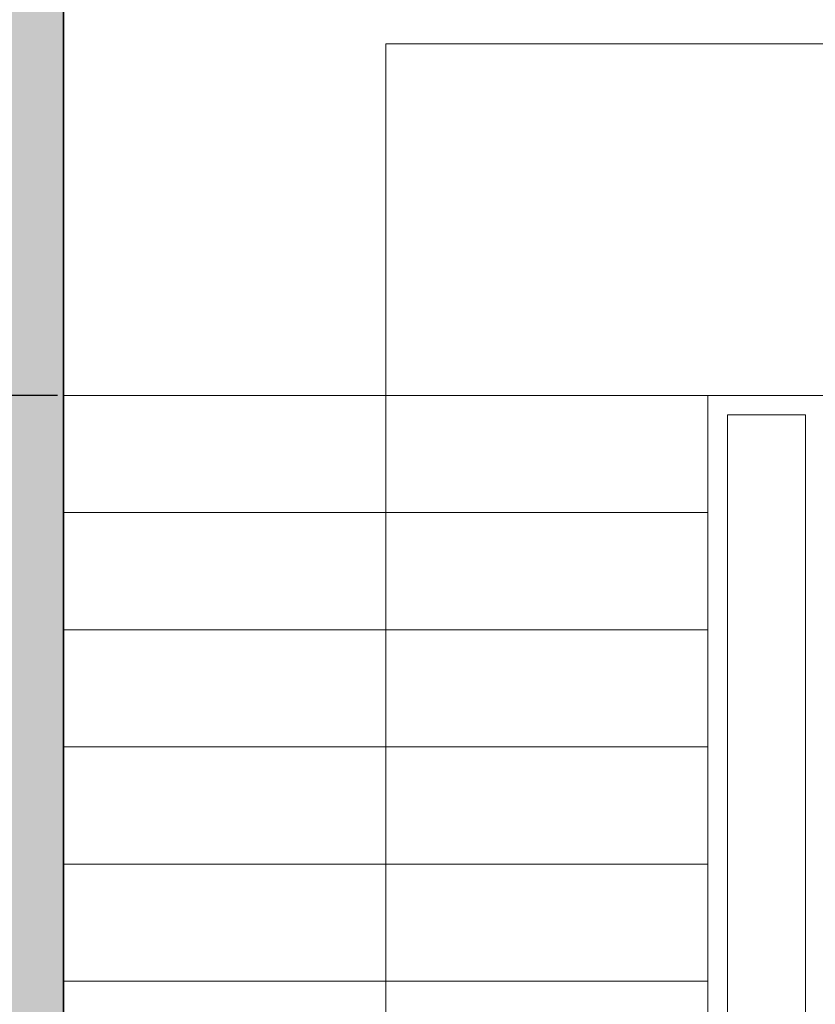
# Model space of a CAD drawing. Units: inches. Extents: x 2083 to 3317, y 1141 to 2115.
# Tile 256 of 256: x 2600 to 2682, y 1877 to 1978. Entities that reach past the tile are written whole.
import ezdxf

# ---------------------------------------------------------------- set-up
doc = ezdxf.new("R2010")
doc.units = ezdxf.units.IN
for name, color, linetype, lineweight in [('A-ANNO-DIMS', 2, 'Continuous', 18), ('A-ANNO-SYMB', 7, 'Continuous', 13), ('A-FLOR-STRS', 7, 'Continuous', 18), ('A-WALL', 7, 'Continuous', 35)]:
    doc.layers.add(name, color=color, linetype=linetype, lineweight=lineweight)
doc.layers.add('A-WALL-PATT', color=251, linetype='Continuous', lineweight=13, true_color=0x636466)
doc.styles.get("Standard").update_dxf_attribs({"font": 'arial.ttf'})
doc.dimstyles.new('ISO-25', dxfattribs={"dimtxt": 12, "dimasz": 12, "dimexe": 1.25, "dimexo": 0.625, "dimtad": 1, "dimlunit": 3, "dimtxsty": 'Standard', "dimcen": 2.5, "dimadec": 0, "dimazin": 0, "dimtfac": 1, "dimtmove": 0, "dimatfit": 3, "dimfxl": 1, "dimarcsym": 0})

# ---------------------------------------------------------------- blocks, each defined once
blk = doc.blocks.new('*D50')
at = {"layer": 'A-ANNO-DIMS', "color": 0, "lineweight": -2, "transparency": 16777216}
for p, q in [((2604.33, 1939.76), (2551.36, 1939.76)), ((2552.61, 1807.76), (2552.61, 1927.76)), ((2604.33, 1795.76), (2551.36, 1795.76))]:
    blk.add_line(p, q, dxfattribs=at)
at = {"layer": 'A-ANNO-DIMS', "color": 0, "transparency": 16777216}
for points in [[(2550.61, 1927.76), (2554.61, 1927.76), (2552.61, 1939.76)], [(2550.61, 1807.76), (2554.61, 1807.76), (2552.61, 1795.76)]]:
    blk.add_solid(points, dxfattribs=at)
at = {"layer": 'Defpoints', "color": 0, "transparency": 16777216}
for p in [(2552.61, 1939.76), (2604.96, 1939.76), (2604.96, 1795.76)]:
    blk.add_point(p, dxfattribs=at)
at = {"layer": 'A-ANNO-DIMS', "color": 0, "transparency": 16777216, "insert": (2545.86, 1867.76), "char_height": 12, "attachment_point": 5, "rotation": 90}
blk.add_mtext('12\'-0"', dxfattribs=at)
blk = doc.blocks.new('*D51')
at = {"layer": 'A-ANNO-DIMS', "color": 0, "lineweight": -2, "transparency": 16777216}
for p, q in [((2604.33, 2011.76), (2551.36, 2011.76)), ((2552.61, 1951.76), (2552.61, 1999.76)), ((2604.33, 1939.76), (2551.36, 1939.76))]:
    blk.add_line(p, q, dxfattribs=at)
at = {"layer": 'A-ANNO-DIMS', "color": 0, "transparency": 16777216}
for points in [[(2550.61, 1999.76), (2554.61, 1999.76), (2552.61, 2011.76)], [(2550.61, 1951.76), (2554.61, 1951.76), (2552.61, 1939.76)]]:
    blk.add_solid(points, dxfattribs=at)
at = {"layer": 'Defpoints', "color": 0, "transparency": 16777216}
for p in [(2552.61, 2011.76), (2604.96, 2011.76), (2604.96, 1939.76)]:
    blk.add_point(p, dxfattribs=at)
at = {"layer": 'A-ANNO-DIMS', "color": 0, "transparency": 16777216, "insert": (2545.86, 1975.76), "char_height": 12, "attachment_point": 5, "rotation": 90}
blk.add_mtext('6\'-0"', dxfattribs=at)

msp = doc.modelspace()

# ---------------------------------------------------------------- hatches: boundary and pattern name
at = {"layer": 'A-WALL-PATT'}
h = msp.add_hatch(color=256, dxfattribs=at)
h.dxf.hatch_style = 1
h.paths.add_polyline_path([(3126.96, 2020.761), (2748.96, 2020.761), (2604.96, 2020.761), (2226.96, 2020.761), (2226.96, 1702.761), (2466.96, 1702.761), (2466.96, 1582.761), (2418.96, 1582.761), (2418.96, 1477.761), (2226.96, 1477.761), (2226.96, 1263.261), (2544.96, 1263.261), (2544.96, 1411.761), (2604.96, 1411.761), (2685.96, 1411.761), (2685.96, 1420.761), (2604.96, 1420.761), (2604.96, 1573.761), (2604.96, 1702.761), (2604.96, 2011.761), (2748.96, 2011.761), (2748.96, 1702.761), (2862.96, 1702.761), (2862.96, 1621.761), (2871.96, 1621.761), (2871.96, 1702.761), (2883.96, 1702.761), (2883.96, 1706.939, -0.0264593), (2883.96, 1711.761), (2757.96, 1711.761), (2757.96, 1807.761), (2787.96, 1807.761), (2787.96, 1812.261), (2757.96, 1812.261), (2757.96, 2011.761), (2877.96, 2011.761), (2877.96, 1812.261), (2847.96, 1812.261), (2847.96, 1807.761), (2889.836, 1807.761), (2889.836, 1812.261), (2882.46, 1812.261), (2882.46, 2011.761), (3117.96, 2011.761), (3117.96, 1812.261), (2937.836, 1812.261), (2937.836, 1807.761), (2995.71, 1807.761), (2995.71, 1796.118), (3000.21, 1796.118), (3000.21, 1807.761), (3117.96, 1807.761), (3117.96, 1711.761), (3000.21, 1711.761), (3000.21, 1760.118), (2998.573, 1760.118, -0.020711), (2995.71, 1760.118), (2995.71, 1711.761), (2931.96, 1711.761), (2931.96, 1702.761), (3126.96, 1702.761)])
h.paths.add_polyline_path([(2471.46, 2011.761), (2471.46, 1810.011), (2462.717, 1810.011), (2462.717, 1805.511), (2505.96, 1805.511), (2505.96, 1810.011), (2475.96, 1810.011), (2475.96, 2011.761), (2595.96, 2011.761), (2595.96, 1810.011), (2565.96, 1810.011), (2565.96, 1805.511), (2595.96, 1805.511), (2595.96, 1711.761), (2235.96, 1711.761), (2235.96, 1805.511), (2353.71, 1805.511), (2353.71, 1796.054), (2358.21, 1796.054), (2358.21, 1805.511), (2414.717, 1805.511), (2414.717, 1810.011), (2235.96, 1810.011), (2235.96, 2011.761)], flags=16)
h.paths.add_polyline_path([(2270.205, 1994.61), (2270.205, 1970.61), (2246.205, 1970.61), (2246.205, 1994.61)], flags=0)
edge = h.paths.add_edge_path(flags=0)
edge.add_ellipse((2332.027, 1899.798), major_axis=(-3.043, 3.043), ratio=0.1682525, start_angle=-161.33217, end_angle=-156.30711, ccw=False)
edge.add_ellipse((2333.082, 1898.744), major_axis=(-1.055, 1.055), ratio=0.4535321, start_angle=-123.37102, end_angle=-94.15911)
edge = h.paths.add_edge_path(flags=0)
edge.add_ellipse((2332.027, 1968.876), major_axis=(3.043, 3.043), ratio=0.1682525, start_angle=18.66783, end_angle=23.69289)
edge.add_spline(control_points=[(2332.926, 1970.691), (2332.227, 1970.336), (2330.894, 1969.659), (2328.413, 1970.932), (2327.204, 1967.749), (2324.71, 1969.956), (2322.533, 1967.012), (2320.013, 1971.296), (2317.68, 1968.158), (2316.041, 1967.102), (2315.427, 1966.81)], knot_values=[0, 0, 0, 0, 2.2670587, 4.3245589, 6.6855835, 8.8786411, 11.121502, 14.300359, 17.7552837, 19.732645, 19.732645, 19.732645, 19.732645], degree=3, periodic=0)
edge.add_ellipse((2332.027, 1968.876), major_axis=(3.043, 3.043), ratio=0.1682525, start_angle=18.66783, end_angle=23.69289, ccw=False)
edge.add_ellipse((2333.082, 1969.931), major_axis=(1.055, 1.055), ratio=0.4535321, start_angle=56.62898, end_angle=85.84089, ccw=False)
edge = h.paths.add_edge_path(flags=0)
edge.add_spline(control_points=[(2296.428, 1967.988), (2293.628, 1965.336), (2287.704, 1959.727), (2299.744, 1949.996), (2294.533, 1935.669), (2290.573, 1920.604), (2293.394, 1909.974), (2296.185, 1904.967)], knot_values=[0.0991853, 0.0991853, 0.0991853, 0.0991853, 0.3453009, 0.6198217, 0.9826526, 1.3860932, 1.8105546, 1.8105546, 1.8105546, 1.8105546], degree=3, periodic=0)
edge.add_spline(control_points=[(2296.185, 1904.967), (2297.384, 1902.619), (2298.001, 1901.949), (2298.553, 1901.468)], knot_values=[0.0062457, 0.0062457, 0.0062457, 0.0062457, 0.0554759, 0.0554759, 0.0554759, 0.0554759], degree=3, periodic=0)
edge.add_spline(control_points=[(2298.553, 1901.468), (2297.259, 1900.923), (2295.225, 1900.232), (2293.06, 1900.614), (2292.101, 1900.788), (2292.09, 1900.791)], knot_values=[0.3128349, 0.3128349, 0.3128349, 0.3128349, 0.4017797, 0.4749867, 0.4759027, 0.4759027, 0.4759027, 0.4759027], degree=3, periodic=0)
edge.add_arc((2292.794, 1904.664), 3.937, 215.4209, 259.69818, ccw=False)
edge.add_spline(control_points=[(2289.585, 1902.382), (2289.477, 1902.535), (2289.368, 1902.688), (2289.261, 1902.841)], knot_values=[0.1028719, 0.1028719, 0.1028719, 0.1028719, 0.1168958, 0.1168958, 0.1168958, 0.1168958], degree=3, periodic=0)
edge.add_spline(control_points=[(2289.261, 1902.841), (2288.687, 1902.55), (2287.64, 1902.02), (2285.881, 1901.874), (2283.853, 1901.504), (2281.72, 1899.711), (2278.467, 1899.493), (2276.157, 1901.883), (2272.259, 1899.804), (2267.778, 1901.843), (2262.244, 1900.184), (2257.415, 1901.782), (2254.318, 1900.726), (2253.178, 1900.337)], knot_values=[0, 0, 0, 0, 1.9079767, 3.4771759, 5.261074, 7.9728515, 11.6802485, 13.7179214, 16.9395917, 22.789562, 27.5025027, 33.5952153, 37.1456181, 37.1456181, 37.1456181, 37.1456181], degree=3, periodic=0)
edge.add_line((2253.178, 1900.337), (2250.244, 1902.841))
edge.add_line((2250.244, 1902.841), (2250.244, 1965.833))
edge.add_line((2250.244, 1965.833), (2253.178, 1968.337))
edge.add_spline(control_points=[(2253.178, 1968.337), (2254.318, 1967.948), (2257.415, 1966.892), (2262.244, 1968.49), (2267.778, 1966.831), (2271.527, 1968.537), (2273.876, 1967.828), (2274.207, 1967.728)], knot_values=[0, 0, 0, 0, 0.0901802, 0.2449351, 0.3646438, 0.5132331, 0.5378548, 0.5378548, 0.5378548, 0.5378548], degree=3, periodic=0)
edge.add_arc((2274.353, 1963.793), 3.937, 72.05113, 92.12795, ccw=False)
edge.add_arc((2281.297, 1985.23), 18.596, 252.05113, 288.56572)
edge.add_arc((2292.317, 1956.029), 12.646, 71.02679, 113.77822, ccw=False)
edge = h.paths.add_edge_path(flags=0)
edge.add_spline(control_points=[(2274.899, 1951.856), (2275.066, 1951.617), (2275.233, 1951.377), (2275.398, 1951.136)], knot_values=[1.4099157, 1.4099157, 1.4099157, 1.4099157, 1.4315903, 1.4315903, 1.4315903, 1.4315903], degree=3, periodic=0)
edge.add_spline(control_points=[(2275.398, 1951.136), (2275.792, 1950.562), (2276.179, 1949.984), (2276.546, 1949.397)], knot_values=[1.3582378, 1.3582378, 1.3582378, 1.3582378, 1.4099157, 1.4099157, 1.4099157, 1.4099157], degree=3, periodic=0)
edge.add_line((2276.546, 1949.397), (2277.437, 1947.862))
edge.add_spline(control_points=[(2277.437, 1947.862), (2276.304, 1945.673), (2274.64, 1942.427), (2274.632, 1938.094), (2272.799, 1930.852), (2274.356, 1943.897), (2275.948, 1947.923), (2276.546, 1949.397)], knot_values=[0.0056315, 0.0056315, 0.0056315, 0.0056315, 0.1860139, 0.2660015, 0.3570872, 0.5963902, 0.7397317, 0.7397317, 0.7397317, 0.7397317], degree=3, periodic=0)
edge.add_spline(control_points=[(2276.546, 1949.397), (2276.179, 1949.984), (2275.792, 1950.562), (2275.398, 1951.136)], knot_values=[1.3582378, 1.3582378, 1.3582378, 1.3582378, 1.4099157, 1.4099157, 1.4099157, 1.4099157], degree=3, periodic=0)
edge.add_spline(control_points=[(2275.398, 1951.136), (2274.943, 1950.08), (2274.208, 1948.025), (2273.935, 1944.851), (2272.469, 1937.627), (2273.466, 1945.696), (2274.701, 1951.059), (2274.899, 1951.856)], knot_values=[0.1043639, 0.1043639, 0.1043639, 0.1043639, 0.1896363, 0.2696239, 0.3607096, 0.6000126, 0.6446217, 0.6446217, 0.6446217, 0.6446217], degree=3, periodic=0)
h.paths.add_polyline_path([(2269.168, 1963.128, -0.3575267), (2268.171, 1960.976, -0.0925607), (2268.171, 1939.436, -0.3575267), (2269.168, 1937.285, -0.3575267), (2267.016, 1938.282, -0.1647847), (2254.686, 1938.282, -0.3575267), (2252.534, 1937.285, -0.3575267), (2253.531, 1939.436, -0.0925607), (2253.531, 1960.976, -0.3575267), (2252.534, 1963.128, -0.3575267), (2254.686, 1962.131, -0.1647847), (2267.016, 1962.131, -0.3575267)], flags=0)
h.paths.add_polyline_path([(2248.874, 1967.802), (2248.874, 1957.028), (2249.458, 1957.028), (2249.458, 1911.647), (2248.874, 1911.647), (2248.874, 1900.873), (2246.512, 1900.873, 0.1973271), (2244.15, 1902.457), (2244.15, 1966.218, 0.1973271), (2246.512, 1967.802)], flags=0)
h.paths.add_polyline_path([(2269.168, 1931.389, -0.3575267), (2268.171, 1929.238, -0.0925607), (2268.171, 1907.698, -0.3575267), (2269.168, 1905.547, -0.3575267), (2267.016, 1906.544, -0.1647847), (2254.686, 1906.544, -0.3575267), (2252.534, 1905.547, -0.3575267), (2253.531, 1907.698, -0.0925607), (2253.531, 1929.238, -0.3575267), (2252.534, 1931.389, -0.3575267), (2254.686, 1930.392, -0.1647847), (2267.016, 1930.392, -0.3575267)], flags=0)
edge = h.paths.add_edge_path(flags=0)
edge.add_spline(control_points=[(2276.197, 1906.724), (2276.168, 1909.029), (2276.114, 1913.372), (2270.598, 1924.925), (2273.905, 1919.013), (2275.922, 1916.262), (2275.475, 1912.402), (2277.258, 1910.381), (2276.696, 1908.225), (2276.646, 1906.813), (2276.618, 1906.008)], knot_values=[0, 0, 0, 0, 8.6102597, 16.2212739, 18.8430575, 23.8048978, 27.4408283, 29.3561016, 31.2034776, 33.6506866, 33.6506866, 33.6506866, 33.6506866], degree=3, periodic=0)
edge.add_spline(control_points=[(2276.618, 1906.008), (2276.623, 1905.624), (2276.498, 1904.629), (2275.442, 1903.855), (2274.937, 1903.08), (2274.859, 1902.841)], knot_values=[0.1564884, 0.1564884, 0.1564884, 0.1564884, 0.1843975, 0.2313765, 0.2505985, 0.2505985, 0.2505985, 0.2505985], degree=3, periodic=0)
edge.add_line((2274.859, 1902.841), (2276.506, 1902.841))
edge.add_spline(control_points=[(2276.506, 1902.841), (2276.788, 1903.085), (2277.665, 1904.125), (2278.25, 1904.341), (2277.654, 1908.527), (2278.156, 1906.228), (2278.1, 1905.286), (2278.847, 1904.069), (2277.857, 1903.415), (2277.874, 1902.991), (2277.904, 1902.841)], knot_values=[0.0595743, 0.0595743, 0.0595743, 0.0595743, 0.0807529, 0.1037415, 0.1697201, 0.1760361, 0.2071372, 0.2404744, 0.2623409, 0.2736605, 0.2736605, 0.2736605, 0.2736605], degree=3, periodic=0)
edge.add_line((2277.904, 1902.841), (2280.03, 1902.841))
edge.add_spline(control_points=[(2280.03, 1902.841), (2279.888, 1903.088), (2279.499, 1903.982), (2280.152, 1905.939), (2278.104, 1909.658), (2279.762, 1907.185), (2280.328, 1904.875), (2280.485, 1903.49), (2281.463, 1903.249), (2281.758, 1902.936), (2281.834, 1902.841)], knot_values=[0.013856, 0.013856, 0.013856, 0.013856, 0.0348738, 0.0888667, 0.1078792, 0.1267378, 0.158714, 0.1937575, 0.2174868, 0.2267221, 0.2267221, 0.2267221, 0.2267221], degree=3, periodic=0)
edge.add_spline(control_points=[(2281.834, 1902.841), (2281.788, 1902.827), (2281.647, 1902.783), (2281.396, 1902.859), (2281.088, 1902.985), (2280.721, 1903.061), (2280.333, 1903.026), (2280.125, 1902.899), (2280.03, 1902.841)], knot_values=[0, 0, 0, 0, 0.1441304, 0.435517, 0.7492759, 1.1530457, 1.5483707, 1.878348, 1.878348, 1.878348, 1.878348], degree=3, periodic=0)
edge.add_line((2280.03, 1902.841), (2277.904, 1902.841))
edge.add_spline(control_points=[(2277.904, 1902.841), (2277.893, 1902.796), (2277.865, 1902.68), (2277.607, 1902.687), (2277.274, 1902.801), (2276.838, 1902.62), (2276.584, 1902.789), (2276.506, 1902.841)], knot_values=[0, 0, 0, 0, 0.1271885, 0.3261988, 0.6280094, 1.2435704, 1.5153306, 1.5153306, 1.5153306, 1.5153306], degree=3, periodic=0)
edge.add_line((2276.506, 1902.841), (2274.859, 1902.841))
edge.add_spline(control_points=[(2274.859, 1902.841), (2274.814, 1902.899), (2274.725, 1903.013), (2274.493, 1903.119), (2274.244, 1902.961), (2273.937, 1903.185), (2273.614, 1902.983), (2273.408, 1902.883), (2273.322, 1902.841)], knot_values=[0, 0, 0, 0, 0.2184302, 0.4369566, 0.6879766, 0.9903786, 1.3983955, 1.6918498, 1.6918498, 1.6918498, 1.6918498], degree=3, periodic=0)
edge.add_spline(control_points=[(2273.322, 1902.841), (2273.617, 1903.446), (2274.274, 1904.538), (2276.027, 1904.574), (2276.207, 1906.584), (2276.197, 1906.724)], knot_values=[0.0122268, 0.0122268, 0.0122268, 0.0122268, 0.0594721, 0.1062177, 0.134458, 0.134458, 0.134458, 0.134458], degree=3, periodic=0)
h.paths.add_polyline_path([(2270.776, 1897.79), (2270.776, 1873.79), (2246.776, 1873.79), (2246.776, 1897.79)], flags=0)
h.paths.add_polyline_path([(2353.71, 1760.005), (2353.71, 1760.054), (2358.21, 1760.054, -0.033729)], flags=0)
h.paths.add_polyline_path([(2321.819, 1737.529), (2341.995, 1737.529, -0.4142136), (2343.203, 1736.321), (2343.203, 1721.021, -0.4142136), (2341.995, 1719.813), (2321.819, 1719.813, -0.4142136), (2320.611, 1721.021), (2320.611, 1736.321, -0.4142136)], flags=0)
h.paths.add_polyline_path([(2324.235, 1736.321), (2339.579, 1736.321, -0.4142136), (2341.995, 1733.905), (2341.995, 1725.45, -0.4142136), (2339.579, 1723.034), (2333.681, 1723.034), (2333.845, 1722.045, -0.8706461), (2335.425, 1721.826, -0.767327), (2333.923, 1721.423), (2331.291, 1721.423, -0.767327), (2329.788, 1721.826, -0.8706461), (2331.368, 1722.045), (2331.533, 1723.034), (2324.235, 1723.034, -0.4142136), (2321.819, 1725.45), (2321.819, 1733.905, -0.4142136)], flags=0)
h.paths.add_polyline_path([(2570.484, 1928.615), (2589.684, 1928.615), (2590.169, 1928.615), (2590.169, 1904.993), (2570.484, 1904.993)], flags=0)
h.paths.add_polyline_path([(2574.447, 1927.264, -1), (2572.829, 1927.264, -1)], flags=0)
h.paths.add_polyline_path([(2573.09, 1926.941), (2573.925, 1927.776), (2574.148, 1927.553), (2573.313, 1926.718)], flags=0)
h.paths.add_polyline_path([(2578.779, 1919.73, -1), (2571.592, 1919.73, -1)], flags=0)
h.paths.add_polyline_path([(2578.385, 1919.73, -1), (2571.985, 1919.73, -1)], flags=0)
h.paths.add_polyline_path([(2331.596, 1729.476, -1), (2333.618, 1729.476, -1)], flags=0)
h.paths.add_polyline_path([(2578.034, 1927.264, -1), (2576.416, 1927.264, -1)], flags=0)
h.paths.add_polyline_path([(2576.689, 1927.531), (2576.912, 1927.754), (2577.747, 1926.919), (2577.524, 1926.696)], flags=0)
h.paths.add_polyline_path([(2578.139, 1909.86, -1), (2572.232, 1909.86, -1)], flags=0)
h.paths.add_polyline_path([(2577.745, 1909.86, -1), (2572.625, 1909.86, -1)], flags=0)
h.paths.add_polyline_path([(2583.798, 1927.264, -1), (2582.179, 1927.264, -1)], flags=0)
h.paths.add_polyline_path([(2582.719, 1927.754), (2583.554, 1926.919), (2583.331, 1926.696), (2582.496, 1927.531)], flags=0)
h.paths.add_polyline_path([(2582.496, 1927.531), (2582.719, 1927.754), (2583.554, 1926.919), (2583.331, 1926.696)], flags=0)
h.paths.add_polyline_path([(2587.739, 1920.53, -1), (2581.832, 1920.53, -1)], flags=0)
h.paths.add_polyline_path([(2587.345, 1920.53, -1), (2582.225, 1920.53, -1)], flags=0)
h.paths.add_polyline_path([(2587.385, 1927.264, -1), (2585.766, 1927.264, -1)], flags=0)
h.paths.add_polyline_path([(2586.082, 1926.98), (2586.917, 1927.815), (2587.14, 1927.593), (2586.305, 1926.758)], flags=0)
h.paths.add_polyline_path([(2588.379, 1910.66, -1), (2581.192, 1910.66, -1)], flags=0)
h.paths.add_polyline_path([(2587.985, 1910.66, -1), (2581.585, 1910.66, -1)], flags=0)
h.paths.add_polyline_path([(2417.168, 1729.478), (2437.344, 1729.478, -0.4142136), (2438.552, 1728.27), (2438.552, 1712.969, -0.4142136), (2437.344, 1711.761), (2417.168, 1711.761, -0.4142136), (2415.96, 1712.969), (2415.96, 1728.27, -0.4142136)], flags=0)
h.paths.add_polyline_path([(2419.584, 1728.27), (2434.928, 1728.27, -0.4142136), (2437.344, 1725.854), (2437.344, 1717.398, -0.4142136), (2434.928, 1714.983), (2429.029, 1714.983), (2429.194, 1713.994, -0.8706461), (2430.774, 1713.775, -0.767327), (2429.271, 1713.372), (2426.64, 1713.372, -0.767327), (2425.137, 1713.775, -0.8706461), (2426.717, 1713.994), (2426.882, 1714.983), (2419.584, 1714.983, -0.4142136), (2417.168, 1717.398), (2417.168, 1725.854, -0.4142136)], flags=0)
h.paths.add_polyline_path([(2419.584, 1728.27), (2434.928, 1728.27, -0.4142136), (2437.344, 1725.854), (2437.344, 1717.398, -0.4142136), (2434.928, 1714.983), (2429.029, 1714.983), (2428.358, 1719.009), (2427.553, 1719.009), (2426.882, 1714.983), (2419.584, 1714.983, -0.4142136), (2417.168, 1717.398), (2417.168, 1725.854, -0.4142136)], flags=0)
h.paths.add_polyline_path([(2426.944, 1721.425, -1), (2428.967, 1721.425, -1)], flags=0)
h.paths.add_polyline_path([(2475.96, 1702.761), (2595.96, 1702.761), (2595.96, 1582.761), (2475.96, 1582.761)], flags=16)
h.paths.add_polyline_path([(2427.96, 1573.761), (2595.96, 1573.761), (2595.96, 1468.761), (2595.96, 1420.761), (2384.46, 1420.761), (2384.46, 1468.761), (2427.96, 1468.761)], flags=16)
h.paths.add_polyline_path([(2379.96, 1468.761), (2379.96, 1420.761), (2235.96, 1420.761), (2235.96, 1468.761)], flags=16)
h.paths.add_polyline_path([(2317.816, 1466.696), (2337.992, 1466.696, -0.4142136), (2339.2, 1465.488), (2339.2, 1450.187, -0.4142136), (2337.992, 1448.979), (2317.816, 1448.979, -0.4142136), (2316.608, 1450.187), (2316.608, 1465.488, -0.4142136)], flags=0)
h.paths.add_polyline_path([(2320.232, 1465.488), (2335.576, 1465.488, -0.4142136), (2337.992, 1463.072), (2337.992, 1454.616, -0.4142136), (2335.576, 1452.2), (2329.677, 1452.2), (2329.842, 1451.212, -0.8706461), (2331.422, 1450.992, -0.767327), (2329.92, 1450.59), (2327.288, 1450.59, -0.767327), (2325.785, 1450.992, -0.8706461), (2327.365, 1451.212), (2327.53, 1452.2), (2320.232, 1452.2, -0.4142136), (2317.816, 1454.616), (2317.816, 1463.072, -0.4142136)], flags=0)
h.paths.add_polyline_path([(2320.232, 1465.488), (2335.576, 1465.488, -0.4142136), (2337.992, 1463.072), (2337.992, 1454.616, -0.4142136), (2335.576, 1452.2), (2329.677, 1452.2), (2329.006, 1456.227), (2328.201, 1456.227), (2327.53, 1452.2), (2320.232, 1452.2, -0.4142136), (2317.816, 1454.616), (2317.816, 1463.072, -0.4142136)], flags=0)
h.paths.add_polyline_path([(2327.593, 1458.643, -1), (2329.615, 1458.643, -1)], flags=0)
h.paths.add_polyline_path([(2244.412, 1433.34), (2241.921, 1433.34, -0.4142136), (2240.018, 1435.244), (2240.018, 1440.953, -0.4142105), (2241.921, 1442.856), (2244.412, 1442.856, -1.9764724)], flags=0)
h.paths.add_polyline_path([(2245.357, 1434.398, -0.4142136), (2245.357, 1441.799, -2.1440985)], flags=0)
h.paths.add_polyline_path([(2535.96, 1416.261), (2535.96, 1272.261), (2235.96, 1272.261), (2235.96, 1416.261)], flags=16)
h.paths.add_polyline_path([(2260.12, 1384.293), (2260.12, 1362.039), (2237.865, 1362.039), (2237.865, 1384.293)], flags=0)
edge = h.paths.add_edge_path(flags=0)
edge.add_line((2318.252, 1362.093), (2318.146, 1362.001))
edge.add_ellipse((2317.445, 1360.431), major_axis=(2.822, 2.822), ratio=0.1682525, start_angle=18.66783, end_angle=20.94813, ccw=False)
edge.add_ellipse((2318.423, 1361.409), major_axis=(0.978, 0.978), ratio=0.4535321, start_angle=56.62898, end_angle=70.2262, ccw=False)
edge = h.paths.add_edge_path(flags=0)
edge.add_line((2319.107, 1295.571), (2319.015, 1295.677))
edge.add_ellipse((2317.445, 1296.378), major_axis=(-2.822, 2.822), ratio=0.1682525, start_angle=-161.33217, end_angle=-159.05187, ccw=False)
edge.add_ellipse((2318.423, 1295.4), major_axis=(-0.978, 0.978), ratio=0.4535321, start_angle=-123.37102, end_angle=-109.7738)
edge = h.paths.add_edge_path(flags=0)
edge.add_spline(control_points=[(2284.21, 1301.17), (2284.581, 1300.445), (2284.891, 1299.892), (2285.16, 1299.461)], knot_values=[0.0390658, 0.0390658, 0.0390658, 0.0390658, 0.0554759, 0.0554759, 0.0554759, 0.0554759], degree=3, periodic=0)
edge.add_line((2285.16, 1299.461), (2284.21, 1301.17))
edge = h.paths.add_edge_path(flags=0)
edge.add_line((2280.412, 1297.298), (2283.37, 1297.036))
edge.add_line((2283.37, 1297.036), (2286.406, 1297.926))
edge.add_spline(control_points=[(2286.406, 1297.926), (2285.305, 1297.463), (2284.345, 1297.129), (2283.37, 1297.036)], knot_values=[0.3943688, 0.3943688, 0.3943688, 0.3943688, 0.4759027, 0.4759027, 0.4759027, 0.4759027], degree=3, periodic=0)
edge.add_spline(control_points=[(2283.37, 1297.036), (2283.281, 1297.028), (2282.316, 1296.957), (2281.313, 1297.134), (2280.423, 1297.296), (2280.412, 1297.298)], knot_values=[0.3128349, 0.3128349, 0.3128349, 0.3128349, 0.3202458, 0.3934528, 0.3943688, 0.3943688, 0.3943688, 0.3943688], degree=3, periodic=0)
edge = h.paths.add_edge_path(flags=0)
edge.add_line((2284.436, 1359.607), (2280.446, 1355.328))
edge.add_line((2280.446, 1355.328), (2279.58, 1351.018))
edge.add_line((2279.58, 1351.018), (2282.413, 1346.58))
edge.add_spline(control_points=[(2282.413, 1346.58), (2283.153, 1345.589), (2284.253, 1344.029), (2284.801, 1342.387), (2284.935, 1341.806)], knot_values=[1.2400982, 1.2400982, 1.2400982, 1.2400982, 1.3328922, 1.3827123, 1.3827123, 1.3827123, 1.3827123], degree=3, periodic=0)
edge.add_spline(control_points=[(2284.935, 1341.806), (2285.319, 1340.141), (2285.233, 1338.409), (2284.91, 1336.654)], knot_values=[1.0974841, 1.0974841, 1.0974841, 1.0974841, 1.2400982, 1.2400982, 1.2400982, 1.2400982], degree=3, periodic=0)
edge.add_spline(control_points=[(2284.91, 1336.654), (2284.587, 1334.899), (2284.027, 1333.12), (2283.463, 1331.361)], knot_values=[0.9548699, 0.9548699, 0.9548699, 0.9548699, 1.0974841, 1.0974841, 1.0974841, 1.0974841], degree=3, periodic=0)
edge.add_line((2283.463, 1331.361), (2281.89, 1326.153))
edge.add_line((2281.89, 1326.153), (2280.756, 1321.056))
edge.add_line((2280.756, 1321.056), (2280.299, 1316.002))
edge.add_line((2280.299, 1316.002), (2280.716, 1310.95))
edge.add_line((2280.716, 1310.95), (2282.028, 1305.972))
edge.add_line((2282.028, 1305.972), (2284.21, 1301.17))
edge.add_spline(control_points=[(2284.21, 1301.17), (2283.341, 1302.73), (2282.612, 1304.336), (2282.028, 1305.972)], knot_values=[0.0991853, 0.0991853, 0.0991853, 0.0991853, 0.2417994, 0.2417994, 0.2417994, 0.2417994], degree=3, periodic=0)
edge.add_spline(control_points=[(2282.028, 1305.972), (2281.444, 1307.608), (2281.005, 1309.273), (2280.716, 1310.95)], knot_values=[0.2417994, 0.2417994, 0.2417994, 0.2417994, 0.3844135, 0.3844135, 0.3844135, 0.3844135], degree=3, periodic=0)
edge.add_spline(control_points=[(2280.716, 1310.95), (2280.433, 1312.588), (2280.289, 1314.277), (2280.299, 1315.962), (2280.299, 1316.002)], knot_values=[0.3844135, 0.3844135, 0.3844135, 0.3844135, 0.5236467, 0.5270276, 0.5270276, 0.5270276, 0.5270276], degree=3, periodic=0)
edge.add_spline(control_points=[(2280.299, 1316.002), (2280.312, 1317.687), (2280.478, 1319.368), (2280.756, 1321.056)], knot_values=[0.5270276, 0.5270276, 0.5270276, 0.5270276, 0.6696417, 0.6696417, 0.6696417, 0.6696417], degree=3, periodic=0)
edge.add_spline(control_points=[(2280.756, 1321.056), (2281.035, 1322.744), (2281.426, 1324.44), (2281.89, 1326.153)], knot_values=[0.6696417, 0.6696417, 0.6696417, 0.6696417, 0.8122558, 0.8122558, 0.8122558, 0.8122558], degree=3, periodic=0)
edge.add_spline(control_points=[(2281.89, 1326.153), (2282.264, 1327.533), (2282.788, 1329.262), (2283.353, 1331.018), (2283.463, 1331.361)], knot_values=[0.8122558, 0.8122558, 0.8122558, 0.8122558, 0.9270873, 0.9548699, 0.9548699, 0.9548699, 0.9548699], degree=3, periodic=0)
edge.add_line((2283.463, 1331.361), (2284.91, 1336.654))
edge.add_line((2284.91, 1336.654), (2284.935, 1341.806))
edge.add_line((2284.935, 1341.806), (2282.413, 1346.58))
edge.add_spline(control_points=[(2282.413, 1346.58), (2281.275, 1348.104), (2280.078, 1349.57), (2279.58, 1351.018)], knot_values=[1.3827123, 1.3827123, 1.3827123, 1.3827123, 1.5253264, 1.5253264, 1.5253264, 1.5253264], degree=3, periodic=0)
edge.add_spline(control_points=[(2279.58, 1351.018), (2279.443, 1351.415), (2279.136, 1352.857), (2279.735, 1354.29), (2280.446, 1355.328)], knot_values=[1.5253264, 1.5253264, 1.5253264, 1.5253264, 1.564439, 1.6679405, 1.6679405, 1.6679405, 1.6679405], degree=3, periodic=0)
edge.add_spline(control_points=[(2280.446, 1355.328), (2281.426, 1356.758), (2282.931, 1358.183), (2284.436, 1359.607)], knot_values=[1.6679405, 1.6679405, 1.6679405, 1.6679405, 1.8105546, 1.8105546, 1.8105546, 1.8105546], degree=3, periodic=0)
edge.add_arc((2280.623, 1348.518), 11.726, 71.02679, 113.77822)
edge.add_arc((2270.405, 1375.595), 17.244, 252.05113, 288.56572, ccw=False)
edge.add_arc((2263.966, 1355.718), 3.651, 72.05113, 92.12795)
edge.add_arc((2263.966, 1355.718), 3.651, 92.12795, 177.98513)
edge.add_spline(control_points=[(2260.318, 1355.846), (2260.26, 1354.221), (2260.551, 1350.187), (2262.999, 1346.766), (2264.473, 1344.649)], knot_values=[1.4315903, 1.4315903, 1.4315903, 1.4315903, 1.5641438, 1.7706953, 1.7706953, 1.7706953, 1.7706953], degree=3, periodic=0)
edge.add_line((2264.473, 1344.649), (2264.936, 1343.983))
edge.add_spline(control_points=[(2263.801, 1340.248), (2263.843, 1340.514), (2264.067, 1341.756), (2264.513, 1343.002), (2264.935, 1343.981)], knot_values=[0.5365702, 0.5365702, 0.5365702, 0.5365702, 0.5593494, 0.6446217, 0.6446217, 0.6446217, 0.6446217], degree=3, periodic=0)
edge.add_spline(control_points=[(2264.935, 1343.981), (2265.118, 1343.715), (2265.299, 1343.448), (2265.477, 1343.179)], knot_values=[1.3840767, 1.3840767, 1.3840767, 1.3840767, 1.4099157, 1.4099157, 1.4099157, 1.4099157], degree=3, periodic=0)
edge.add_spline(control_points=[(2265.477, 1343.179), (2265.655, 1342.911), (2265.829, 1342.641), (2265.999, 1342.369)], knot_values=[1.3582378, 1.3582378, 1.3582378, 1.3582378, 1.3840767, 1.3840767, 1.3840767, 1.3840767], degree=3, periodic=0)
edge.add_line((2265.999, 1342.369), (2266.826, 1340.946))
edge.add_spline(control_points=[(2266.826, 1340.946), (2268.894, 1337.09), (2271.398, 1325.843), (2270.516, 1310.569), (2275.919, 1301.861), (2277.79, 1299.199)], knot_values=[0.1168958, 0.1168958, 0.1168958, 0.1168958, 0.4729873, 1.0509689, 1.3137934, 1.3137934, 1.3137934, 1.3137934], degree=3, periodic=0)
edge.add_spline(control_points=[(2277.79, 1299.199), (2277.839, 1299.128), (2277.889, 1299.057), (2277.94, 1298.987)], knot_values=[0.1098839, 0.1098839, 0.1098839, 0.1098839, 0.1168958, 0.1168958, 0.1168958, 0.1168958], degree=3, periodic=0)
edge.add_line((2277.94, 1298.987), (2277.789, 1299.199))
edge.add_spline(control_points=[(2277.789, 1299.199), (2277.257, 1298.929), (2276.286, 1298.438), (2275.039, 1298.334), (2274.383, 1298.239), (2274.215, 1298.209)], knot_values=[33.1218702, 33.1218702, 33.1218702, 33.1218702, 35.0290557, 36.5982549, 37.1448269, 37.1448269, 37.1448269, 37.1448269], degree=3, periodic=0)
edge.add_line((2274.215, 1298.209), (2273.073, 1297.893))
edge.add_spline(control_points=[(2273.073, 1297.893), (2272.323, 1297.58), (2271.039, 1296.511), (2269.248, 1296.226), (2268.423, 1296.375)], knot_values=[26.5325843, 26.5325843, 26.5325843, 26.5325843, 29.198919, 31.8391012, 31.8391012, 31.8391012, 31.8391012], degree=3, periodic=0)
edge.add_line((2268.423, 1296.375), (2263.879, 1297.458))
edge.add_spline(control_points=[(2263.879, 1297.458), (2263.556, 1297.359), (2261.86, 1296.839), (2260.239, 1297.282), (2258.933, 1297.516)], knot_values=[15.9195506, 15.9195506, 15.9195506, 15.9195506, 16.9395917, 21.2260675, 21.2260675, 21.2260675, 21.2260675], degree=3, periodic=0)
edge.add_line((2258.933, 1297.516), (2254.055, 1297.329))
edge.add_spline(control_points=[(2254.055, 1297.329), (2253.756, 1297.296), (2252.114, 1297.165), (2250.462, 1297.544), (2249.13, 1297.668)], knot_values=[5.3065169, 5.3065169, 5.3065169, 5.3065169, 6.2764352, 10.6130337, 10.6130337, 10.6130337, 10.6130337], degree=3, periodic=0)
edge.add_line((2249.13, 1297.668), (2244.332, 1296.878))
edge.add_line((2244.332, 1296.878), (2241.611, 1299.199))
edge.add_line((2241.611, 1299.199), (2241.611, 1357.609))
edge.add_line((2241.611, 1357.609), (2244.332, 1359.931))
edge.add_line((2244.332, 1359.931), (2252.729, 1359.543))
edge.add_spline(control_points=[(2252.729, 1359.543), (2252.871, 1359.546), (2253.306, 1359.548), (2253.74, 1359.514), (2254.032, 1359.482)], knot_values=[0.233291, 0.233291, 0.233291, 0.233291, 0.2449351, 0.2689274, 0.2689274, 0.2689274, 0.2689274], degree=3, periodic=0)
edge.add_line((2254.032, 1359.482), (2259.587, 1359.416))
edge.add_spline(control_points=[(2259.587, 1359.416), (2260.677, 1359.629), (2262.073, 1359.897), (2263.524, 1359.459), (2263.83, 1359.366)], knot_values=[0.4225164, 0.4225164, 0.4225164, 0.4225164, 0.5132331, 0.5378548, 0.5378548, 0.5378548, 0.5378548], degree=3, periodic=0)
edge.add_arc((2263.966, 1355.718), 3.651, 72.05113, 92.12795, ccw=False)
edge.add_arc((2270.405, 1375.595), 17.244, 252.05113, 288.56572)
edge.add_arc((2280.623, 1348.518), 11.726, 71.02679, 113.77822, ccw=False)
h.paths.add_polyline_path([(2240.341, 1359.435), (2240.341, 1349.444), (2240.882, 1349.444), (2240.882, 1307.365), (2240.341, 1307.365), (2240.341, 1297.374), (2238.15, 1297.374, 0.1973271), (2235.96, 1298.843), (2235.96, 1357.966, 0.1973271), (2238.15, 1359.435)], flags=0)
h.paths.add_polyline_path([(2259.158, 1355.101, -0.3575267), (2258.233, 1353.106, -0.0925607), (2258.233, 1333.133, -0.3575267), (2259.158, 1331.138, -0.3575267), (2257.163, 1332.062, -0.1647847), (2245.729, 1332.062, -0.3575267), (2243.735, 1331.138, -0.3575267), (2244.659, 1333.133, -0.0925607), (2244.659, 1353.106, -0.3575267), (2243.735, 1355.101, -0.3575267), (2245.729, 1354.176, -0.1647847), (2257.163, 1354.176, -0.3575267)], flags=0)
edge = h.paths.add_edge_path(flags=0)
edge.add_line((2265.999, 1342.369), (2266.826, 1340.946))
edge.add_line((2266.826, 1340.946), (2265.308, 1337.814))
edge.add_line((2265.308, 1337.814), (2264.358, 1334.653))
edge.add_line((2264.358, 1334.653), (2264.262, 1333.8))
edge.add_spline(control_points=[(2264.262, 1333.8), (2264.208, 1333.187), (2264.162, 1332.366), (2264.007, 1331.414), (2263.969, 1331.202)], knot_values=[0.4644442, 0.4644442, 0.4644442, 0.4644442, 0.5166905, 0.5316081, 0.5316081, 0.5316081, 0.5316081], degree=3, periodic=0)
edge.add_spline(control_points=[(2263.969, 1331.202), (2263.775, 1330.119), (2263.424, 1328.791), (2263.257, 1328.531), (2263.234, 1328.515)], knot_values=[0.3726816, 0.3726816, 0.3726816, 0.3726816, 0.4488497, 0.4644442, 0.4644442, 0.4644442, 0.4644442], degree=3, periodic=0)
edge.add_spline(control_points=[(2263.234, 1328.515), (2263.096, 1328.42), (2263.131, 1329.301), (2263.275, 1330.616)], knot_values=[0.2809191, 0.2809191, 0.2809191, 0.2809191, 0.3726816, 0.3726816, 0.3726816, 0.3726816], degree=3, periodic=0)
edge.add_spline(control_points=[(2263.275, 1330.616), (2263.419, 1331.93), (2263.672, 1333.677), (2263.97, 1335.315)], knot_values=[0.1891566, 0.1891566, 0.1891566, 0.1891566, 0.2809191, 0.2809191, 0.2809191, 0.2809191], degree=3, periodic=0)
edge.add_spline(control_points=[(2263.97, 1335.315), (2264.1, 1336.032), (2264.419, 1337.622), (2264.755, 1338.864), (2264.947, 1339.491)], knot_values=[0.097394, 0.097394, 0.097394, 0.097394, 0.1375775, 0.1891566, 0.1891566, 0.1891566, 0.1891566], degree=3, periodic=0)
edge.add_spline(control_points=[(2264.947, 1339.491), (2265.29, 1340.606), (2265.644, 1341.494), (2265.999, 1342.369)], knot_values=[0.0056315, 0.0056315, 0.0056315, 0.0056315, 0.097394, 0.097394, 0.097394, 0.097394], degree=3, periodic=0)
h.paths.add_polyline_path([(2259.158, 1325.671, -0.3575267), (2258.233, 1323.676, -0.0925607), (2258.233, 1303.703, -0.3575267), (2259.158, 1301.708, -0.3575267), (2257.163, 1302.633, -0.1647847), (2245.729, 1302.633, -0.3575267), (2243.735, 1301.708, -0.3575267), (2244.659, 1303.703, -0.0925607), (2244.659, 1323.676, -0.3575267), (2243.735, 1325.671, -0.3575267), (2245.729, 1324.747, -0.1647847), (2257.163, 1324.747, -0.3575267)], flags=0)
edge = h.paths.add_edge_path(flags=0)
edge.add_spline(control_points=[(2261.709, 1317.311), (2261.679, 1317.418), (2261.762, 1317.389), (2262.491, 1316.09), (2262.962, 1315.301)], knot_values=[14.9558607, 14.9558607, 14.9558607, 14.9558607, 16.2212739, 18.6948259, 18.6948259, 18.6948259, 18.6948259], degree=3, periodic=0)
edge.add_spline(control_points=[(2262.962, 1315.301), (2262.99, 1315.254), (2263.702, 1314.067), (2264.349, 1313.127), (2264.73, 1312.164)], knot_values=[18.6948259, 18.6948259, 18.6948259, 18.6948259, 18.8430575, 22.433791, 22.433791, 22.433791, 22.433791], degree=3, periodic=0)
edge.add_spline(control_points=[(2264.73, 1312.164), (2264.876, 1311.796), (2265.177, 1310.77), (2265.143, 1309.559), (2265.248, 1308.824)], knot_values=[22.433791, 22.433791, 22.433791, 22.433791, 23.8048978, 26.1727562, 26.1727562, 26.1727562, 26.1727562], degree=3, periodic=0)
edge.add_line((2265.248, 1308.824), (2265.851, 1307.172))
edge.add_spline(control_points=[(2265.851, 1307.172), (2266.065, 1306.822), (2266.384, 1306.332), (2266.424, 1305.781), (2266.42, 1305.611)], knot_values=[28.0625624, 28.0625624, 28.0625624, 28.0625624, 29.3561016, 29.9117214, 29.9117214, 29.9117214, 29.9117214], degree=3, periodic=0)
edge.add_spline(control_points=[(2266.42, 1305.611), (2266.416, 1305.433), (2266.394, 1305.25), (2266.365, 1305.066)], knot_values=[29.9117214, 29.9117214, 29.9117214, 29.9117214, 30.4978371, 30.4978371, 30.4978371, 30.4978371], degree=3, periodic=0)
edge.add_line((2266.365, 1305.066), (2266.066, 1302.136))
edge.add_spline(control_points=[(2266.066, 1302.136), (2266.071, 1301.78), (2265.998, 1301.2), (2265.663, 1300.759), (2265.509, 1300.586)], knot_values=[0.1564884, 0.1564884, 0.1564884, 0.1564884, 0.1843975, 0.2035434, 0.2035434, 0.2035434, 0.2035434], degree=3, periodic=0)
edge.add_line((2265.509, 1300.586), (2264.435, 1299.199))
edge.add_line((2264.435, 1299.199), (2265.962, 1299.199))
edge.add_line((2265.962, 1299.199), (2267.336, 1301.175))
edge.add_line((2267.336, 1301.175), (2267.312, 1301.986))
edge.add_spline(control_points=[(2267.312, 1301.986), (2267.261, 1302.862), (2267.16, 1303.737), (2267.271, 1303.326)], knot_values=[0.1262286, 0.1262286, 0.1262286, 0.1262286, 0.1666174, 0.1666174, 0.1666174, 0.1666174], degree=3, periodic=0)
edge.add_spline(control_points=[(2267.271, 1303.326), (2267.28, 1303.294), (2267.31, 1303.175), (2267.373, 1302.884), (2267.406, 1302.683), (2267.418, 1302.601)], knot_values=[0.1666174, 0.1666174, 0.1666174, 0.1666174, 0.1697201, 0.1760361, 0.1807647, 0.1807647, 0.1807647, 0.1807647], degree=3, periodic=0)
edge.add_spline(control_points=[(2267.744, 1300.988), (2267.688, 1301.151), (2267.481, 1301.657), (2267.484, 1302.145), (2267.418, 1302.601)], knot_values=[0.1807647, 0.1807647, 0.1807647, 0.1807647, 0.1937665, 0.2201389, 0.2201389, 0.2201389, 0.2201389], degree=3, periodic=0)
edge.add_line((2267.418, 1302.601), (2267.744, 1300.988))
edge.add_spline(control_points=[(2267.744, 1300.988), (2267.832, 1300.732), (2267.932, 1300.31), (2267.555, 1299.975), (2267.429, 1299.829)], knot_values=[0.2201389, 0.2201389, 0.2201389, 0.2201389, 0.2404744, 0.2548903, 0.2548903, 0.2548903, 0.2548903], degree=3, periodic=0)
edge.add_line((2267.429, 1299.829), (2267.258, 1299.199))
edge.add_line((2267.258, 1299.199), (2269.23, 1299.199))
edge.add_spline(control_points=[(2269.23, 1299.199), (2269.099, 1299.429), (2268.843, 1300.016), (2269.012, 1300.916), (2268.947, 1301.661)], knot_values=[0.013856, 0.013856, 0.013856, 0.013856, 0.0348738, 0.0670726, 0.0670726, 0.0670726, 0.0670726], degree=3, periodic=0)
edge.add_line((2268.947, 1301.661), (2268.432, 1303.603))
edge.add_spline(control_points=[(2268.432, 1303.603), (2268.176, 1304.192), (2267.596, 1305.251), (2268.041, 1304.623), (2268.251, 1304.282)], knot_values=[0.0901547, 0.0901547, 0.0901547, 0.0901547, 0.1078792, 0.1202891, 0.1202891, 0.1202891, 0.1202891], degree=3, periodic=0)
edge.add_spline(control_points=[(2268.251, 1304.282), (2268.361, 1304.105), (2269.058, 1302.918), (2269.383, 1301.59), (2269.521, 1300.776), (2269.575, 1300.556)], knot_values=[0.1202891, 0.1202891, 0.1202891, 0.1202891, 0.1267378, 0.158714, 0.1735056, 0.1735056, 0.1735056, 0.1735056], degree=3, periodic=0)
edge.add_line((2269.575, 1300.556), (2270.686, 1299.421))
edge.add_spline(control_points=[(2270.686, 1299.421), (2270.767, 1299.357), (2270.838, 1299.281), (2270.903, 1299.199)], knot_values=[0.2181597, 0.2181597, 0.2181597, 0.2181597, 0.2267221, 0.2267221, 0.2267221, 0.2267221], degree=3, periodic=0)
edge.add_line((2270.937, 1299.193), (2270.903, 1299.199))
edge.add_spline(control_points=[(2270.903, 1299.199), (2270.86, 1299.186), (2270.73, 1299.146), (2270.496, 1299.216), (2270.272, 1299.308), (2270.121, 1299.348), (2270.063, 1299.36)], knot_values=[0.939174, 0.939174, 0.939174, 0.939174, 1.0833044, 1.3746911, 1.6884499, 1.878348, 1.878348, 1.878348, 1.878348], degree=3, periodic=0)
edge.add_line((2270.063, 1299.36), (2269.23, 1299.199))
edge.add_line((2269.23, 1299.199), (2267.258, 1299.199))
edge.add_spline(control_points=[(2267.258, 1299.199), (2267.248, 1299.157), (2267.223, 1299.05), (2266.984, 1299.057), (2266.809, 1299.116), (2266.677, 1299.109), (2266.637, 1299.105)], knot_values=[0.7576653, 0.7576653, 0.7576653, 0.7576653, 0.8848538, 1.0838641, 1.3856747, 1.5153306, 1.5153306, 1.5153306, 1.5153306], degree=3, periodic=0)
edge.add_spline(control_points=[(2266.637, 1299.105), (2266.485, 1299.089), (2266.236, 1299.017), (2266.035, 1299.151), (2265.962, 1299.199)], knot_values=[0, 0, 0, 0, 0.4859051, 0.7576653, 0.7576653, 0.7576653, 0.7576653], degree=3, periodic=0)
edge.add_line((2265.962, 1299.199), (2264.435, 1299.199))
edge.add_line((2264.435, 1299.199), (2263.858, 1299.367))
edge.add_spline(control_points=[(2263.858, 1299.367), (2263.819, 1299.371), (2263.78, 1299.386), (2263.74, 1299.402)], knot_values=[0.8459249, 0.8459249, 0.8459249, 0.8459249, 0.9786272, 0.9786272, 0.9786272, 0.9786272], degree=3, periodic=0)
edge.add_line((2263.722, 1299.396), (2263.01, 1299.199))
edge.add_spline(control_points=[(2263.01, 1299.199), (2263.246, 1299.683), (2263.506, 1300.128), (2263.873, 1300.408)], knot_values=[0.0122268, 0.0122268, 0.0122268, 0.0122268, 0.0529705, 0.0529705, 0.0529705, 0.0529705], degree=3, periodic=0)
edge.add_spline(control_points=[(2263.873, 1300.408), (2263.932, 1300.453), (2264.084, 1300.553), (2264.255, 1300.624), (2264.36, 1300.665)], knot_values=[0.0529705, 0.0529705, 0.0529705, 0.0529705, 0.0594721, 0.0690861, 0.0690861, 0.0690861, 0.0690861], degree=3, periodic=0)
edge.add_line((2264.36, 1300.665), (2265.142, 1301.078))
edge.add_line((2265.142, 1301.078), (2265.676, 1302.8))
edge.add_line((2265.676, 1302.8), (2265.541, 1305.704))
edge.add_line((2265.541, 1305.704), (2264.803, 1309.328))
edge.add_line((2264.803, 1309.328), (2263.041, 1314.092))
edge.add_spline(control_points=[(2263.041, 1314.092), (2262.384, 1315.671), (2261.796, 1316.998), (2261.709, 1317.311)], knot_values=[11.2168955, 11.2168955, 11.2168955, 11.2168955, 14.9558607, 14.9558607, 14.9558607, 14.9558607], degree=3, periodic=0)
h.paths.add_polyline_path([(2871.96, 1416.261), (2895.91, 1416.261), (2895.91, 1420.761), (2871.96, 1420.761), (2871.96, 1501.761), (2862.96, 1501.761), (2862.96, 1420.761), (2805.96, 1420.761), (2805.96, 1411.761), (2862.96, 1411.761), (2862.96, 1263.261), (3126.96, 1263.261), (3126.96, 1411.761), (3126.96, 1486.761), (2943.96, 1486.761), (2943.96, 1477.761), (2967.86, 1477.761), (2967.86, 1420.761), (2943.91, 1420.761), (2943.91, 1416.261), (3117.96, 1416.261), (3117.96, 1420.761), (2972.36, 1420.761), (2972.36, 1477.761), (3117.96, 1477.761), (3117.96, 1420.761), (3117.96, 1272.261), (2871.96, 1272.261)], flags=0)
h.paths.add_polyline_path([(2457.126, 1485.943), (2527.603, 1485.943), (2527.603, 1537.636), (2457.126, 1537.636)], flags=8)
h.paths.add_polyline_path([(2481.005, 1609.982), (2590.766, 1609.982), (2590.766, 1682.003), (2481.005, 1682.003)], flags=8)
h.paths.add_polyline_path([(2483.085, 1729.127), (2553.562, 1729.127), (2553.562, 1780.82), (2483.085, 1780.82)], flags=8)

# ---------------------------------------------------------------- linework, layer by layer
at = {"layer": 'A-ANNO-SYMB'}
for q in [(2637.96, 1795.761), (2715.96, 1975.761)]:
    msp.add_line((2637.96, 1975.761), q, dxfattribs=at)
at = {"layer": 'A-FLOR-STRS'}
for p, q in [((2604.96, 1939.761), (2748.96, 1939.761)), ((2670.96, 1939.761), (2670.96, 1795.761)), ((2672.96, 1937.761), (2680.96, 1937.761)), ((2672.96, 1937.761), (2672.96, 1797.761)), ((2680.96, 1937.761), (2680.96, 1797.761)), ((2604.96, 1927.761), (2670.96, 1927.761)), ((2604.96, 1915.761), (2670.96, 1915.761)), ((2604.96, 1903.761), (2670.96, 1903.761)), ((2604.96, 1891.761), (2670.96, 1891.761)), ((2604.96, 1879.761), (2670.96, 1879.761))]:
    msp.add_line(p, q, dxfattribs=at)
at = {"layer": 'A-WALL'}
msp.add_line((2604.96, 2011.761), (2604.96, 1702.761), dxfattribs=at)

# ---------------------------------------------------------------- dimensions: what is measured, and where the dimension line sits
at = {"layer": 'A-ANNO-DIMS'}
for base, p1, p2, picture, middle in [((2552.61, 2011.761), (2604.96, 1939.761), (2604.96, 2011.761), '*D51', (2545.858, 1975.761)), ((2552.61, 1939.761), (2604.96, 1795.761), (2604.96, 1939.761), '*D50', (2545.858, 1867.761))]:
    dim = msp.add_linear_dim(base=base, p1=p1, p2=p2, angle=90, dimstyle='ISO-25', override={"dimdec": 1, "dimlfac": 1, "dimrnd": 0, "dimzin": 1, "dimdsep": 46, "dimlunit": 4, "dimfrac": 2}, dxfattribs=at)
    dim.commit()
    dim.dimension.update_dxf_attribs({"geometry": picture, "text_midpoint": middle})

doc.saveas('drawing.dxf')
